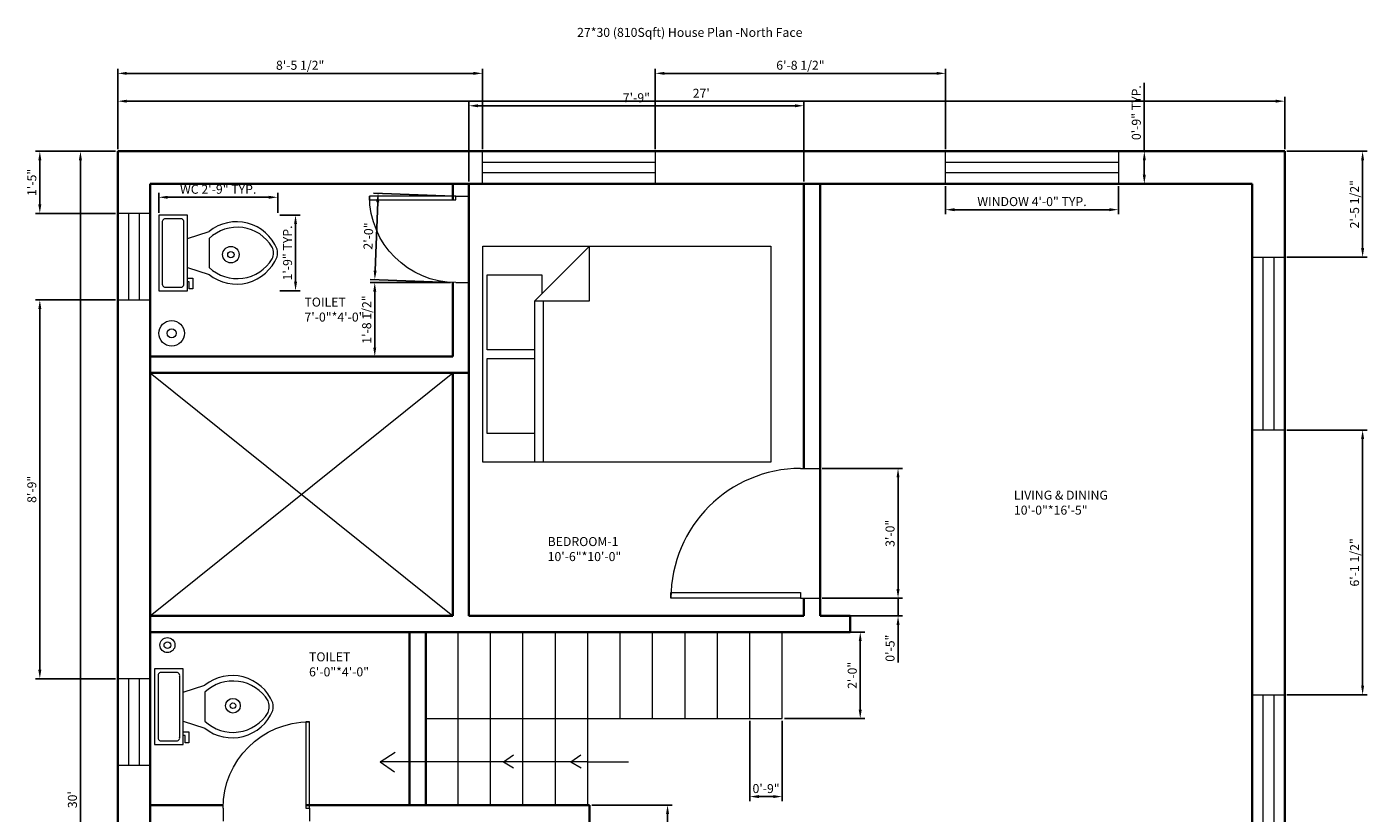
# Model space of a CAD drawing. Units: inches. Extents: x 2721 to 3093, y 1944 to 2371.
# Tile 2 of 2: x 2721 to 3093, y 2152 to 2371. Entities that reach past the tile are written whole.
import ezdxf

# ---------------------------------------------------------------- set-up
doc = ezdxf.new("R2010")
doc.units = ezdxf.units.IN
for name, color, linetype, lineweight in [('A-ANNO-DIMS', 2, 'Continuous', 18), ('A-ANNO-SYMB', 7, 'Continuous', 13), ('A-ANNO-TEXT', 7, 'Continuous', 18), ('A-AREA-IDEN', 7, 'Continuous', 18), ('A-DOOR', 3, 'Continuous', 18), ('A-FLOR-FIXT', 8, 'Continuous', 18), ('A-FLOR-OPEN', 8, 'Continuous', 13), ('A-FLOR-STRS', 7, 'Continuous', 20), ('A-FURN', 9, 'Continuous', 18), ('A-GLAZ', 4, 'Continuous', 18), ('A-WALL', 7, 'Continuous', 35)]:
    doc.layers.add(name, color=color, linetype=linetype, lineweight=lineweight)
doc.styles.get("Standard").update_dxf_attribs({"font": 'arial.ttf'})
doc.dimstyles.new('ISO-25', dxfattribs={"dimtxt": 2.5, "dimasz": 2.5, "dimexe": 1.25, "dimexo": 0.625, "dimtad": 1, "dimdec": 1, "dimlunit": 3, "dimtxsty": 'Standard', "dimcen": 2.5, "dimadec": 0, "dimazin": 0, "dimtfac": 1, "dimtdec": 1, "dimtmove": 0, "dimatfit": 3, "dimfxl": 1, "dimarcsym": 0})

# ---------------------------------------------------------------- blocks, each defined once
blk = doc.blocks.new('*U2')
for p, q in [((0, 0), (0, -6)), ((40, 0), (40, -6))]:
    blk.add_line(p, q)
blk.add_lwpolyline([(0, 0), (0, 40), (1.75, 40), (1.75, 0)], close=True)
blk.add_arc((0, 0), 40, 0, 90)
blk = doc.blocks.new('Bed - Queen')
for p, q in [((0, -80.00003), (0, 0)), ((0, 0), (59.99999, 0)), ((59.99999, 0), (59.99999, -80.00003)), ((7.99999, -1.2), (28.79998, -1.2)), ((7.99999, -14.4), (7.99999, -1.2)), ((28.79998, -1.2), (28.79998, -14.4)), ((31.19999, -1.2), (51.99999, -1.2)), ((31.19999, -14.4), (31.19999, -1.2)), ((51.99999, -1.2), (51.99999, -16.4)), ((0, -14.4), (44.8, -14.4)), ((59.99999, -29.6), (44.8, -14.4)), ((44.8, -14.4), (44.8, -29.6)), ((44.8, -16.8), (0, -16.8)), ((51.99999, -16.4), (46.79936, -16.4)), ((44.8, -29.6), (59.99999, -29.6)), ((59.99999, -80.00003), (0, -80.00003))]:
    blk.add_line(p, q)
blk = doc.blocks.new('Toilet - top')
for p, q in [((9.5, -6), (9.5, -2)), ((-10, -8.5), (-8, -8.5)), ((-10, -9.5), (-10, -8.5)), ((-7, -9.5), (-10, -9.5)), ((-8, -8.5), (-8, -8)), ((-7, -8), (-7, -9.5)), ((-4, -8), (-6, -14)), ((4, -8), (6, -14)), ((4, -14), (-4, -14))]:
    blk.add_line(p, q)
blk.add_lwpolyline([(10.5, -8), (10.5, 0), (-10.5, 0), (-10.5, -8)], close=True)
for points in [[(-9.5, -2), (-9.5, -6)], [(8.5, -1), (-8.5, -1)], [(-8.5, -7), (8.5, -7)]]:
    blk.add_lwpolyline(points)
for centre, radius, start, end in [((-8.62, -1.88), 0.884, 81.8699, 188.1301), ((8.62, -1.88), 0.884, 351.8699, 98.1301), ((-8.62, -6.12), 0.884, 171.8699, 278.1301), ((8.62, -6.12), 0.884, 261.8699, 8.1301), ((3.52, -21.58), 12.17, 141.4691, 247.9714), ((4.2, -21.82), 11.33, 136.3677, 238.9468), ((-3.52, -21.58), 12.17, 292.0284, 38.5307), ((-4.2, -21.82), 11.33, 301.053, 43.6321), ((0, -27.88), 4, 245.7318, 294.2682), ((0, -29), 4, 254.8605, 285.1395)]:
    blk.add_arc(centre, radius, start, end)
blk = doc.blocks.new('*D6')
at = {"layer": 'A-ANNO-DIMS', "color": 0, "lineweight": -2, "transparency": 16777216}
for p, q in [((2745.8, 2336.8), (2745.8, 2351.35)), ((2748.3, 2350.1), (3067.3, 2350.1)), ((3069.8, 2336.8), (3069.8, 2351.35))]:
    blk.add_line(p, q, dxfattribs=at)
at = {"layer": 'A-ANNO-DIMS', "color": 0, "transparency": 16777216}
for points in [[(2748.3, 2350.52), (2748.3, 2349.69), (2745.8, 2350.1)], [(3067.3, 2350.52), (3067.3, 2349.69), (3069.8, 2350.1)]]:
    blk.add_solid(points, dxfattribs=at)
at = {"layer": 'Defpoints', "color": 0, "transparency": 16777216}
for p in [(3069.8, 2350.1), (2745.8, 2336.18), (3069.8, 2336.18)]:
    blk.add_point(p, dxfattribs=at)
at = {"layer": 'A-ANNO-DIMS', "color": 0, "transparency": 16777216, "insert": (2907.8, 2351.98), "char_height": 2.5, "attachment_point": 5}
blk.add_mtext("27'", dxfattribs=at)
blk = doc.blocks.new('*D7')
at = {"layer": 'A-ANNO-DIMS', "color": 0, "lineweight": -2, "transparency": 16777216}
for p, q in [((2745.17, 2336.18), (2734.17, 2336.18)), ((2735.42, 2333.68), (2735.42, 1978.68)), ((2745.17, 1976.18), (2734.17, 1976.18))]:
    blk.add_line(p, q, dxfattribs=at)
at = {"layer": 'A-ANNO-DIMS', "color": 0, "transparency": 16777216}
for points in [[(2735, 2333.68), (2735.84, 2333.68), (2735.42, 2336.18)], [(2735, 1978.68), (2735.84, 1978.68), (2735.42, 1976.18)]]:
    blk.add_solid(points, dxfattribs=at)
at = {"layer": 'Defpoints', "color": 0, "transparency": 16777216}
for p in [(2745.8, 2336.18), (2735.42, 1976.18), (2745.8, 1976.18)]:
    blk.add_point(p, dxfattribs=at)
at = {"layer": 'A-ANNO-DIMS', "color": 0, "transparency": 16777216, "insert": (2733.52, 2156.18), "char_height": 2.5, "attachment_point": 5, "rotation": 90}
blk.add_mtext("30'", dxfattribs=at)
blk = doc.blocks.new('WIN-48IN')
for p, q in [((0, 9), (48, 9)), ((0, 0), (0, 9)), ((48, 9), (48, 0)), ((0, 6), (48, 6)), ((48, 3), (0, 3)), ((48, 0), (0, 0))]:
    blk.add_line(p, q)
blk = doc.blocks.new('WIN-24IN')
for p, q in [((9, 24), (0, 24)), ((0, 24), (0, 0)), ((3, 24), (3, 0)), ((6, 0), (6, 24)), ((9, 0), (9, 24)), ((0, 0), (9, 0))]:
    blk.add_line(p, q)
blk = doc.blocks.new('*D11')
at = {"layer": 'A-ANNO-DIMS', "color": 0, "lineweight": -2, "transparency": 16777216}
for p, q in [((2975.63, 2326.55), (2975.63, 2318.73)), ((3023.63, 2326.55), (3023.63, 2318.73)), ((2978.13, 2319.98), (3021.13, 2319.98))]:
    blk.add_line(p, q, dxfattribs=at)
at = {"layer": 'A-ANNO-DIMS', "color": 0, "transparency": 16777216}
for points in [[(2978.13, 2320.39), (2978.13, 2319.56), (2975.63, 2319.98)], [(3021.13, 2320.39), (3021.13, 2319.56), (3023.63, 2319.98)]]:
    blk.add_solid(points, dxfattribs=at)
at = {"layer": 'Defpoints', "color": 0, "transparency": 16777216}
for p in [(2975.63, 2327.18), (3023.63, 2327.18), (3023.63, 2319.98)]:
    blk.add_point(p, dxfattribs=at)
at = {"layer": 'A-ANNO-DIMS', "color": 0, "transparency": 16777216, "insert": (2999.63, 2321.9), "char_height": 2.5, "attachment_point": 5}
blk.add_mtext('WINDOW 4\'-0" TYP.', dxfattribs=at)
blk = doc.blocks.new('*D12')
at = {"layer": 'A-ANNO-DIMS', "color": 0, "lineweight": -2, "transparency": 16777216}
for p, q in [((3030.83, 2336.18), (3030.83, 2355.17)), ((3024.26, 2336.18), (3032.08, 2336.18)), ((3030.83, 2329.68), (3030.83, 2333.68)), ((3024.26, 2327.18), (3032.08, 2327.18))]:
    blk.add_line(p, q, dxfattribs=at)
at = {"layer": 'A-ANNO-DIMS', "color": 0, "transparency": 16777216}
for points in [[(3030.41, 2333.68), (3031.25, 2333.68), (3030.83, 2336.18)], [(3030.41, 2329.68), (3031.25, 2329.68), (3030.83, 2327.18)]]:
    blk.add_solid(points, dxfattribs=at)
at = {"layer": 'Defpoints', "color": 0, "transparency": 16777216}
for p in [(3023.63, 2336.18), (3030.83, 2336.18), (3023.63, 2327.18)]:
    blk.add_point(p, dxfattribs=at)
at = {"layer": 'A-ANNO-DIMS', "color": 0, "transparency": 16777216, "insert": (3028.93, 2346.92), "char_height": 2.5, "attachment_point": 5, "rotation": 90}
blk.add_mtext('0\'-9" TYP.', dxfattribs=at)
blk = doc.blocks.new('*D17')
at = {"layer": 'A-ANNO-DIMS', "color": 0, "lineweight": -2, "transparency": 16777216}
for p, q in [((2757.15, 2319.09), (2757.15, 2324.67)), ((2787.69, 2323.42), (2759.65, 2323.42)), ((2790.19, 2319.09), (2790.19, 2324.67))]:
    blk.add_line(p, q, dxfattribs=at)
at = {"layer": 'A-ANNO-DIMS', "color": 0, "transparency": 16777216}
for points in [[(2759.65, 2323.83), (2759.65, 2323), (2757.15, 2323.42)], [(2787.69, 2323.83), (2787.69, 2323), (2790.19, 2323.42)]]:
    blk.add_solid(points, dxfattribs=at)
at = {"layer": 'Defpoints', "color": 0, "transparency": 16777216}
for p in [(2757.15, 2323.42), (2757.15, 2318.46), (2790.19, 2318.46)]:
    blk.add_point(p, dxfattribs=at)
at = {"layer": 'A-ANNO-DIMS', "color": 0, "transparency": 16777216, "insert": (2773.67, 2325.33), "char_height": 2.5, "attachment_point": 5}
blk.add_mtext('WC 2\'-9" TYP.', dxfattribs=at)
blk = doc.blocks.new('*D18')
at = {"layer": 'A-ANNO-DIMS', "color": 0, "lineweight": -2, "transparency": 16777216}
for p, q in [((2790.82, 2318.46), (2796.4, 2318.46)), ((2795.15, 2299.96), (2795.15, 2315.96)), ((2790.82, 2297.46), (2796.4, 2297.46))]:
    blk.add_line(p, q, dxfattribs=at)
at = {"layer": 'A-ANNO-DIMS', "color": 0, "transparency": 16777216}
for points in [[(2794.74, 2315.96), (2795.57, 2315.96), (2795.15, 2318.46)], [(2794.74, 2299.96), (2795.57, 2299.96), (2795.15, 2297.46)]]:
    blk.add_solid(points, dxfattribs=at)
at = {"layer": 'Defpoints', "color": 0, "transparency": 16777216}
for p in [(2790.19, 2318.46), (2795.15, 2318.46), (2790.19, 2297.46)]:
    blk.add_point(p, dxfattribs=at)
at = {"layer": 'A-ANNO-DIMS', "color": 0, "transparency": 16777216, "insert": (2793.25, 2307.96), "char_height": 2.5, "attachment_point": 5, "rotation": 90}
blk.add_mtext('1\'-9" TYP.', dxfattribs=at)
blk = doc.blocks.new('*D23')
at = {"layer": 'A-ANNO-DIMS', "color": 0, "lineweight": -2, "transparency": 16777216}
for p, q in [((2745.8, 2336.8), (2745.8, 2359.08)), ((2748.3, 2357.83), (2844.55, 2357.83)), ((2847.05, 2336.8), (2847.05, 2359.08))]:
    blk.add_line(p, q, dxfattribs=at)
at = {"layer": 'A-ANNO-DIMS', "color": 0, "transparency": 16777216}
for points in [[(2748.3, 2358.24), (2748.3, 2357.41), (2745.8, 2357.83)], [(2844.55, 2358.24), (2844.55, 2357.41), (2847.05, 2357.83)]]:
    blk.add_solid(points, dxfattribs=at)
at = {"layer": 'Defpoints', "color": 0, "transparency": 16777216}
for p in [(2847.05, 2357.83), (2745.8, 2336.18), (2847.05, 2336.18)]:
    blk.add_point(p, dxfattribs=at)
at = {"layer": 'A-ANNO-DIMS', "color": 0, "transparency": 16777216, "insert": (2796.43, 2359.75), "char_height": 2.5, "attachment_point": 5}
blk.add_mtext('8\'-5 1/2"', dxfattribs=at)
blk = doc.blocks.new('*D24')
at = {"layer": 'A-ANNO-DIMS', "color": 0, "lineweight": -2, "transparency": 16777216}
for p, q in [((2895.05, 2336.8), (2895.05, 2359.08)), ((2897.55, 2357.83), (2973.13, 2357.83)), ((2975.63, 2336.8), (2975.63, 2359.08))]:
    blk.add_line(p, q, dxfattribs=at)
at = {"layer": 'A-ANNO-DIMS', "color": 0, "transparency": 16777216}
for points in [[(2897.55, 2358.24), (2897.55, 2357.41), (2895.05, 2357.83)], [(2973.13, 2358.24), (2973.13, 2357.41), (2975.63, 2357.83)]]:
    blk.add_solid(points, dxfattribs=at)
at = {"layer": 'Defpoints', "color": 0, "transparency": 16777216}
for p in [(2975.63, 2357.83), (2895.05, 2336.18), (2975.63, 2336.18)]:
    blk.add_point(p, dxfattribs=at)
at = {"layer": 'A-ANNO-DIMS', "color": 0, "transparency": 16777216, "insert": (2935.34, 2359.75), "char_height": 2.5, "attachment_point": 5}
blk.add_mtext('6\'-8 1/2"', dxfattribs=at)
blk = doc.blocks.new('*D28')
at = {"layer": 'A-ANNO-DIMS', "color": 0, "lineweight": -2, "transparency": 16777216}
for p, q in [((2745.17, 2336.18), (2722.9, 2336.18)), ((2724.15, 2321.43), (2724.15, 2333.68)), ((2745.17, 2318.93), (2722.9, 2318.93))]:
    blk.add_line(p, q, dxfattribs=at)
at = {"layer": 'A-ANNO-DIMS', "color": 0, "transparency": 16777216}
for points in [[(2723.73, 2333.68), (2724.56, 2333.68), (2724.15, 2336.18)], [(2723.73, 2321.43), (2724.56, 2321.43), (2724.15, 2318.93)]]:
    blk.add_solid(points, dxfattribs=at)
at = {"layer": 'Defpoints', "color": 0, "transparency": 16777216}
for p in [(2724.15, 2336.18), (2745.8, 2336.18), (2745.8, 2318.93)]:
    blk.add_point(p, dxfattribs=at)
at = {"layer": 'A-ANNO-DIMS', "color": 0, "transparency": 16777216, "insert": (2722.25, 2327.56), "char_height": 2.5, "attachment_point": 5, "rotation": 90}
blk.add_mtext('1\'-5"', dxfattribs=at)
blk = doc.blocks.new('*D29')
at = {"layer": 'A-ANNO-DIMS', "color": 0, "lineweight": -2, "transparency": 16777216}
for p, q in [((2745.17, 2294.93), (2722.9, 2294.93)), ((2724.15, 2192.23), (2724.15, 2292.43)), ((2745.17, 2189.73), (2722.9, 2189.73))]:
    blk.add_line(p, q, dxfattribs=at)
at = {"layer": 'A-ANNO-DIMS', "color": 0, "transparency": 16777216}
for points in [[(2723.73, 2292.43), (2724.56, 2292.43), (2724.15, 2294.93)], [(2723.73, 2192.23), (2724.56, 2192.23), (2724.15, 2189.73)]]:
    blk.add_solid(points, dxfattribs=at)
at = {"layer": 'Defpoints', "color": 0, "transparency": 16777216}
for p in [(2724.15, 2294.93), (2745.8, 2294.93), (2745.8, 2189.73)]:
    blk.add_point(p, dxfattribs=at)
at = {"layer": 'A-ANNO-DIMS', "color": 0, "transparency": 16777216, "insert": (2722.25, 2242.33), "char_height": 2.5, "attachment_point": 5, "rotation": 90}
blk.add_mtext('8\'-9"', dxfattribs=at)
blk = doc.blocks.new('*D30')
at = {"layer": 'A-ANNO-DIMS', "color": 0, "lineweight": -2, "transparency": 16777216}
for p, q in [((3070.42, 2336.18), (3092.7, 2336.18)), ((3091.45, 2333.68), (3091.45, 2309.3)), ((3070.42, 2306.8), (3092.7, 2306.8))]:
    blk.add_line(p, q, dxfattribs=at)
at = {"layer": 'A-ANNO-DIMS', "color": 0, "transparency": 16777216}
for points in [[(3091.03, 2333.68), (3091.86, 2333.68), (3091.45, 2336.18)], [(3091.03, 2309.3), (3091.86, 2309.3), (3091.45, 2306.8)]]:
    blk.add_solid(points, dxfattribs=at)
at = {"layer": 'Defpoints', "color": 0, "transparency": 16777216}
for p in [(3069.8, 2336.18), (3069.8, 2306.8), (3091.45, 2306.8)]:
    blk.add_point(p, dxfattribs=at)
at = {"layer": 'A-ANNO-DIMS', "color": 0, "transparency": 16777216, "insert": (3089.53, 2321.49), "char_height": 2.5, "attachment_point": 5, "rotation": 90}
blk.add_mtext('2\'-5 1/2"', dxfattribs=at)
blk = doc.blocks.new('*D31')
at = {"layer": 'A-ANNO-DIMS', "color": 0, "lineweight": -2, "transparency": 16777216}
for p, q in [((3070.42, 2258.8), (3092.7, 2258.8)), ((3091.45, 2256.3), (3091.45, 2187.81)), ((3070.42, 2185.31), (3092.7, 2185.31))]:
    blk.add_line(p, q, dxfattribs=at)
at = {"layer": 'A-ANNO-DIMS', "color": 0, "transparency": 16777216}
for points in [[(3091.03, 2256.3), (3091.86, 2256.3), (3091.45, 2258.8)], [(3091.03, 2187.81), (3091.86, 2187.81), (3091.45, 2185.31)]]:
    blk.add_solid(points, dxfattribs=at)
at = {"layer": 'Defpoints', "color": 0, "transparency": 16777216}
for p in [(3069.8, 2258.8), (3069.8, 2185.31), (3091.45, 2185.31)]:
    blk.add_point(p, dxfattribs=at)
at = {"layer": 'A-ANNO-DIMS', "color": 0, "transparency": 16777216, "insert": (3089.53, 2222.05), "char_height": 2.5, "attachment_point": 5, "rotation": 90}
blk.add_mtext('6\'-1 1/2"', dxfattribs=at)
blk = doc.blocks.new('*D34')
at = {"layer": 'A-ANNO-DIMS', "color": 0, "lineweight": -2, "transparency": 16777216}
for p, q in [((2930.92, 2202.68), (2953.2, 2202.68)), ((2951.95, 2200.18), (2951.95, 2181.18)), ((2930.92, 2178.68), (2953.2, 2178.68))]:
    blk.add_line(p, q, dxfattribs=at)
at = {"layer": 'A-ANNO-DIMS', "color": 0, "transparency": 16777216}
for points in [[(2951.53, 2200.18), (2952.36, 2200.18), (2951.95, 2202.68)], [(2951.53, 2181.18), (2952.36, 2181.18), (2951.95, 2178.68)]]:
    blk.add_solid(points, dxfattribs=at)
at = {"layer": 'Defpoints', "color": 0, "transparency": 16777216}
for p in [(2930.3, 2202.68), (2930.3, 2178.68), (2951.95, 2178.68)]:
    blk.add_point(p, dxfattribs=at)
at = {"layer": 'A-ANNO-DIMS', "color": 0, "transparency": 16777216, "insert": (2950.05, 2190.68), "char_height": 2.5, "attachment_point": 5, "rotation": 90}
blk.add_mtext('2\'-0"', dxfattribs=at)
blk = doc.blocks.new('*D35')
at = {"layer": 'A-ANNO-DIMS', "color": 0, "lineweight": -2, "transparency": 16777216}
for p, q in [((2921.3, 2178.05), (2921.3, 2155.78)), ((2930.3, 2178.05), (2930.3, 2155.78)), ((2927.8, 2157.03), (2923.8, 2157.03))]:
    blk.add_line(p, q, dxfattribs=at)
at = {"layer": 'A-ANNO-DIMS', "color": 0, "transparency": 16777216}
for points in [[(2923.8, 2157.44), (2923.8, 2156.61), (2921.3, 2157.03)], [(2927.8, 2157.44), (2927.8, 2156.61), (2930.3, 2157.03)]]:
    blk.add_solid(points, dxfattribs=at)
at = {"layer": 'Defpoints', "color": 0, "transparency": 16777216}
for p in [(2921.3, 2178.68), (2930.3, 2178.68), (2921.3, 2157.03)]:
    blk.add_point(p, dxfattribs=at)
at = {"layer": 'A-ANNO-DIMS', "color": 0, "transparency": 16777216, "insert": (2925.8, 2158.93), "char_height": 2.5, "attachment_point": 5}
blk.add_mtext('0\'-9"', dxfattribs=at)
blk = doc.blocks.new('*D36')
at = {"layer": 'A-ANNO-DIMS', "color": 0, "lineweight": -2, "transparency": 16777216}
for p, q in [((2941.42, 2248.12), (2963.7, 2248.12)), ((2962.45, 2245.62), (2962.45, 2214.62)), ((2941.42, 2212.12), (2963.7, 2212.12))]:
    blk.add_line(p, q, dxfattribs=at)
at = {"layer": 'A-ANNO-DIMS', "color": 0, "transparency": 16777216}
for points in [[(2962.03, 2245.62), (2962.86, 2245.62), (2962.45, 2248.12)], [(2962.03, 2214.62), (2962.86, 2214.62), (2962.45, 2212.12)]]:
    blk.add_solid(points, dxfattribs=at)
at = {"layer": 'Defpoints', "color": 0, "transparency": 16777216}
for p in [(2940.8, 2248.12), (2940.8, 2212.12), (2962.45, 2212.12)]:
    blk.add_point(p, dxfattribs=at)
at = {"layer": 'A-ANNO-DIMS', "color": 0, "transparency": 16777216, "insert": (2960.55, 2230.12), "char_height": 2.5, "attachment_point": 5, "rotation": 90}
blk.add_mtext('3\'-0"', dxfattribs=at)
blk = doc.blocks.new('*D43')
at = {"layer": 'A-ANNO-DIMS', "color": 0, "lineweight": -2, "transparency": 16777216}
for p, q in [((2839.07, 2323.76), (2816.81, 2324.6)), ((2817.26, 2303.06), (2817.97, 2322.05)), ((2838.17, 2299.78), (2815.91, 2300.61))]:
    blk.add_line(p, q, dxfattribs=at)
at = {"layer": 'A-ANNO-DIMS', "color": 0, "transparency": 16777216}
for points in [[(2817.55, 2322.07), (2818.39, 2322.04), (2818.06, 2324.55)], [(2816.84, 2303.08), (2817.67, 2303.05), (2817.16, 2300.57)]]:
    blk.add_solid(points, dxfattribs=at)
at = {"layer": 'Defpoints', "color": 0, "transparency": 16777216}
for p in [(2818.06, 2324.55), (2839.7, 2323.74), (2838.8, 2299.75)]:
    blk.add_point(p, dxfattribs=at)
at = {"layer": 'A-ANNO-DIMS', "color": 0, "transparency": 16777216, "insert": (2815.71, 2312.63), "char_height": 2.5, "attachment_point": 5, "rotation": 87.8509}
blk.add_mtext('2\'-0"', dxfattribs=at)
blk = doc.blocks.new('*D44')
at = {"layer": 'A-ANNO-DIMS', "color": 0, "lineweight": -2, "transparency": 16777216}
for p, q in [((2838.17, 2299.75), (2815.9, 2299.75)), ((2817.15, 2281.68), (2817.15, 2297.25)), ((2838.17, 2279.18), (2815.9, 2279.18))]:
    blk.add_line(p, q, dxfattribs=at)
at = {"layer": 'A-ANNO-DIMS', "color": 0, "transparency": 16777216}
for points in [[(2816.73, 2297.25), (2817.56, 2297.25), (2817.15, 2299.75)], [(2816.73, 2281.68), (2817.56, 2281.68), (2817.15, 2279.18)]]:
    blk.add_solid(points, dxfattribs=at)
at = {"layer": 'Defpoints', "color": 0, "transparency": 16777216}
for p in [(2817.15, 2299.75), (2838.8, 2299.75), (2838.8, 2279.18)]:
    blk.add_point(p, dxfattribs=at)
at = {"layer": 'A-ANNO-DIMS', "color": 0, "transparency": 16777216, "insert": (2815.23, 2289.47), "char_height": 2.5, "attachment_point": 5, "rotation": 90}
blk.add_mtext('1\'-8 1/2"', dxfattribs=at)
blk = doc.blocks.new('*D45')
at = {"layer": 'A-ANNO-DIMS', "color": 0, "lineweight": -2, "transparency": 16777216}
for p, q in [((2962.45, 2214.62), (2962.45, 2217.12)), ((2941.42, 2212.12), (2963.7, 2212.12)), ((2962.45, 2212.12), (2962.45, 2207.18)), ((2941.42, 2207.18), (2963.7, 2207.18)), ((2962.45, 2204.68), (2962.45, 2194.28))]:
    blk.add_line(p, q, dxfattribs=at)
at = {"layer": 'A-ANNO-DIMS', "color": 0, "transparency": 16777216}
for points in [[(2962.03, 2214.62), (2962.86, 2214.62), (2962.45, 2212.12)], [(2962.03, 2204.68), (2962.86, 2204.68), (2962.45, 2207.18)]]:
    blk.add_solid(points, dxfattribs=at)
at = {"layer": 'Defpoints', "color": 0, "transparency": 16777216}
for p in [(2940.8, 2212.12), (2940.8, 2207.18), (2962.45, 2207.18)]:
    blk.add_point(p, dxfattribs=at)
at = {"layer": 'A-ANNO-DIMS', "color": 0, "transparency": 16777216, "insert": (2960.55, 2198.23), "char_height": 2.5, "attachment_point": 5, "rotation": 90}
blk.add_mtext('0\'-5"', dxfattribs=at)
blk = doc.blocks.new('*D46')
at = {"layer": 'A-ANNO-DIMS', "color": 0, "lineweight": -2, "transparency": 16777216}
for p, q in [((2877.42, 2154.68), (2899.7, 2154.68)), ((2898.45, 2152.18), (2898.45, 2147.68)), ((2877.42, 2145.18), (2899.7, 2145.18)), ((2898.45, 2145.18), (2898.45, 2128.96))]:
    blk.add_line(p, q, dxfattribs=at)
at = {"layer": 'A-ANNO-DIMS', "color": 0, "transparency": 16777216}
for points in [[(2898.03, 2152.18), (2898.86, 2152.18), (2898.45, 2154.68)], [(2898.03, 2147.68), (2898.86, 2147.68), (2898.45, 2145.18)]]:
    blk.add_solid(points, dxfattribs=at)
at = {"layer": 'Defpoints', "color": 0, "transparency": 16777216}
for p in [(2876.8, 2154.68), (2876.8, 2145.18), (2898.45, 2145.18)]:
    blk.add_point(p, dxfattribs=at)
at = {"layer": 'A-ANNO-DIMS', "color": 0, "transparency": 16777216, "insert": (2896.53, 2135.82), "char_height": 2.5, "attachment_point": 5, "rotation": 90}
blk.add_mtext('0\'-9 1/2"', dxfattribs=at)
blk = doc.blocks.new('*D49')
at = {"layer": 'A-ANNO-DIMS', "color": 0, "lineweight": -2, "transparency": 16777216}
for p, q in [((2843.3, 2327.8), (2843.3, 2350.08)), ((2845.8, 2348.83), (2933.8, 2348.83)), ((2936.3, 2327.8), (2936.3, 2350.08))]:
    blk.add_line(p, q, dxfattribs=at)
at = {"layer": 'A-ANNO-DIMS', "color": 0, "transparency": 16777216}
for points in [[(2845.8, 2349.24), (2845.8, 2348.41), (2843.3, 2348.83)], [(2933.8, 2349.24), (2933.8, 2348.41), (2936.3, 2348.83)]]:
    blk.add_solid(points, dxfattribs=at)
at = {"layer": 'Defpoints', "color": 0, "transparency": 16777216}
for p in [(2936.3, 2348.83), (2843.3, 2327.18), (2936.3, 2327.18)]:
    blk.add_point(p, dxfattribs=at)
at = {"layer": 'A-ANNO-DIMS', "color": 0, "transparency": 16777216, "insert": (2889.8, 2350.73), "char_height": 2.5, "attachment_point": 5}
blk.add_mtext('7\'-9"', dxfattribs=at)

msp = doc.modelspace()

# ---------------------------------------------------------------- linework, layer by layer
at = {"layer": 'A-ANNO-SYMB'}
for p, q in [((2818.66, 2166.68), (2822.83, 2169.35)), ((2876.3, 2166.68), (2818.66, 2166.68)), ((2818.66, 2166.68), (2822.63, 2163.9)), ((2852.92, 2166.68), (2855.68, 2168.64)), ((2852.92, 2166.68), (2855.68, 2165.04)), ((2871.59, 2166.68), (2874.34, 2168.59)), ((2871.59, 2166.68), (2874.47, 2165.02)), ((2876.3, 2166.68), (2887.63, 2166.68))]:
    msp.add_line(p, q, dxfattribs=at)
at = {"layer": 'A-FLOR-FIXT'}
for centre, radius in [((2777.2, 2307.5), 2.29), ((2777.2, 2307.5), 0.886), ((2760.74, 2285.65), 3.55), ((2760.74, 2285.65), 1.28), ((2759.57, 2199.09), 2.09), ((2759.57, 2199.09), 0.925), ((2777.78, 2182.26), 2.04), ((2777.78, 2182.26), 0.773)]:
    msp.add_circle(centre, radius, dxfattribs=at)
at = {"layer": 'A-FLOR-OPEN'}
for p, q in [((2754.8, 2274.68), (2838.8, 2207.18)), ((2754.8, 2207.18), (2838.8, 2274.68))]:
    msp.add_line(p, q, dxfattribs=at)
at = {"layer": 'A-FLOR-STRS'}
for p, q in [((2840.3, 2154.68), (2840.3, 2202.68)), ((2849.3, 2154.68), (2849.3, 2202.68)), ((2858.3, 2154.68), (2858.3, 2202.68)), ((2867.3, 2154.68), (2867.3, 2202.68)), ((2876.3, 2154.68), (2876.3, 2202.68)), ((2885.3, 2178.68), (2885.3, 2202.68)), ((2894.3, 2178.68), (2894.3, 2202.68)), ((2903.3, 2178.68), (2903.3, 2202.68)), ((2912.3, 2178.68), (2912.3, 2202.68)), ((2921.3, 2178.68), (2921.3, 2202.68)), ((2930.3, 2178.68), (2930.3, 2202.68)), ((2831.3, 2178.68), (2930.3, 2178.68))]:
    msp.add_line(p, q, dxfattribs=at)
at = {"layer": 'A-WALL'}
for p, q in [((2745.8, 2336.18), (3069.8, 2336.18)), ((2745.8, 1976.18), (2745.8, 2336.18)), ((3069.8, 2336.18), (3069.8, 1976.18)), ((2754.8, 2327.18), (3060.8, 2327.18)), ((2754.8, 1985.18), (2754.8, 2327.18)), ((2838.8, 2322.69), (2838.8, 2327.18)), ((2843.3, 2207.18), (2843.3, 2327.18)), ((2936.3, 2327.18), (2936.3, 2248.12)), ((2940.8, 2327.18), (2940.8, 2207.18)), ((3060.8, 2327.18), (3060.8, 2130.18)), ((2838.8, 2279.18), (2838.8, 2299.75)), ((2754.8, 2279.18), (2838.8, 2279.18)), ((2754.8, 2274.68), (2843.3, 2274.68)), ((2838.8, 2207.18), (2838.8, 2274.68)), ((2936.3, 2212.12), (2936.3, 2207.18)), ((2754.8, 2207.18), (2838.8, 2207.18)), ((2843.3, 2207.18), (2936.3, 2207.18)), ((2940.8, 2207.18), (2949.18, 2207.18)), ((2949.18, 2202.68), (2949.18, 2207.18)), ((2754.8, 2202.68), (2940.8, 2202.68)), ((2826.8, 2154.68), (2826.8, 2202.68)), ((2831.3, 2154.68), (2831.3, 2202.68)), ((2940.8, 2202.68), (2949.18, 2202.68)), ((2754.8, 2154.68), (2775.04, 2154.68)), ((2797.98, 2154.68), (2876.8, 2154.68)), ((2876.8, 2154.68), (2876.8, 1985.18))]:
    msp.add_line(p, q, dxfattribs=at)

# ---------------------------------------------------------------- block references
at = {"layer": 'A-DOOR'}
for p, xscale, yscale, zscale, rotation in [((2839.7, 2323.74), -0.6, 0.6, 0.6, 90), ((2935.4, 2212.12), 0.9, 0.9, 0.9, 90.00000000000003)]:
    msp.add_blockref('*U2', p, dxfattribs=dict(at, xscale=xscale, yscale=yscale, zscale=zscale, rotation=rotation))
at = {"layer": 'A-DOOR', "xscale": -0.6, "yscale": 0.6, "zscale": 0.6}
msp.add_blockref('*U2', (2799.03, 2153.78), dxfattribs=at)
at = {"layer": 'A-FLOR-FIXT', "rotation": 90}
for p in [(2757.15, 2307.96), (2755.98, 2181.99)]:
    msp.add_blockref('Toilet - top', p, dxfattribs=at)
at = {"layer": 'A-FURN', "rotation": 90}
msp.add_blockref('Bed - Queen', (2847.15, 2249.87), dxfattribs=at)
at = {"layer": 'A-GLAZ'}
for name, p in [('WIN-48IN', (2847.05, 2327.18)), ('WIN-48IN', (2975.63, 2327.18)), ('WIN-24IN', (2745.8, 2294.93)), ('WIN-24IN', (2745.8, 2165.73))]:
    msp.add_blockref(name, p, dxfattribs=at)
for p, rotation in [((3069.8, 2258.8), 90.00000000000317), ((3069.8, 2137.31), 90.00000000000276)]:
    msp.add_blockref('WIN-48IN', p, dxfattribs=dict(at, rotation=rotation))

# ---------------------------------------------------------------- texts
at = {"layer": 'A-ANNO-TEXT', "insert": (2873.33, 2370.45), "char_height": 2.5, "attachment_point": 1}
msp.add_mtext_dynamic_manual_height_columns('27*30 (810Sqft) House Plan -North Face', width=309.6567, gutter_width=12.5, heights=[0], dxfattribs=at)
at = {"layer": 'A-AREA-IDEN', "char_height": 2.5, "attachment_point": 1}
for s, width, insert in [('TOILET\\P7\'-0"*4\'-0"', 45.6593, (2797.63, 2295.57)), ('LIVING & DINING\\P10\'-0"*16\'-5"', 53.9387, (2994.62, 2241.97)), ('BEDROOM-1\\P10\'-6"*10\'-0"', 36.6403, (2865.15, 2229.08)), ('TOILET\\P6\'-0"*4\'-0"', 29.6279, (2798.9, 2197.07))]:
    msp.add_mtext_dynamic_manual_height_columns(s, width=width, gutter_width=12.5, heights=[0], dxfattribs=dict(at, insert=insert))

# ---------------------------------------------------------------- dimensions: what is measured, and where the dimension line sits
at = {"layer": 'A-ANNO-DIMS'}
for base, p1, p2, angle, override, picture, middle in [((2847.054, 2357.8275), (2745.7983, 2336.1775), (2847.054, 2336.1775), 0, {"dimdec": 1, "dimlfac": 1, "dimrnd": 0, "dimzin": 1, "dimdsep": 46, "dimlunit": 4, "dimfrac": 2}, '*D23', (2796.4262, 2359.7451)), ((2724.1483, 2336.1775), (2745.7983, 2318.9347), (2745.7983, 2336.1775), 90, {"dimdec": 1, "dimlfac": 1, "dimrnd": 0, "dimzin": 1, "dimdsep": 46, "dimlunit": 4, "dimfrac": 2}, '*D28', (2722.2469, 2327.5561)), ((2735.42, 1976.18), (2745.8, 2336.18), (2745.8, 1976.18), 90, {"dimclrd": 0, "dimclre": 0, "dimclrt": 0}, '*D7', (2733.52, 2156.18)), ((3091.45, 2306.8), (3069.8, 2336.18), (3069.8, 2306.8), 270, {"dimdec": 1, "dimlfac": 1, "dimrnd": 0, "dimzin": 1, "dimdsep": 46, "dimlunit": 4, "dimfrac": 2}, '*D30', (3089.53, 2321.49)), ((2818.06, 2324.55), (2838.8, 2299.75), (2839.7, 2323.74), 87.8509, {"dimdec": 1, "dimlfac": 1, "dimrnd": 0, "dimzin": 1, "dimdsep": 46, "dimlunit": 4, "dimfrac": 2}, '*D43', (2815.71, 2312.63)), ((2817.15, 2299.75), (2838.8, 2279.18), (2838.8, 2299.75), 90, {"dimdec": 1, "dimlfac": 1, "dimrnd": 0, "dimzin": 1, "dimdsep": 46, "dimlunit": 4, "dimfrac": 2}, '*D44', (2815.23, 2289.47)), ((2724.15, 2294.93), (2745.8, 2189.73), (2745.8, 2294.93), 90, {"dimdec": 1, "dimlfac": 1, "dimrnd": 0, "dimzin": 1, "dimdsep": 46, "dimlunit": 4, "dimfrac": 2}, '*D29', (2722.25, 2242.33)), ((3091.45, 2185.31), (3069.8, 2258.8), (3069.8, 2185.31), 270, {"dimdec": 1, "dimlfac": 1, "dimrnd": 0, "dimzin": 1, "dimdsep": 46, "dimlunit": 4, "dimfrac": 2}, '*D31', (3089.53, 2222.05)), ((2962.45, 2212.12), (2940.8, 2248.12), (2940.8, 2212.12), 270, {"dimdec": 1, "dimlfac": 1, "dimrnd": 0, "dimzin": 1, "dimdsep": 46, "dimlunit": 4, "dimfrac": 2}, '*D36', (2960.55, 2230.12)), ((2962.45, 2207.18), (2940.8, 2212.12), (2940.8, 2207.18), 270, {"dimdec": 1, "dimlfac": 1, "dimrnd": 0, "dimzin": 1, "dimdsep": 46, "dimlunit": 4, "dimfrac": 2}, '*D45', (2960.55, 2198.23)), ((2951.95, 2178.68), (2930.3, 2202.68), (2930.3, 2178.68), 270, {"dimdec": 1, "dimlfac": 1, "dimrnd": 0, "dimzin": 1, "dimdsep": 46, "dimlunit": 4, "dimfrac": 2}, '*D34', (2950.05, 2190.68)), ((2921.3, 2157.03), (2930.3, 2178.68), (2921.3, 2178.68), 180, {"dimdec": 1, "dimlfac": 1, "dimrnd": 0, "dimzin": 1, "dimdsep": 46, "dimlunit": 4, "dimfrac": 2}, '*D35', (2925.8, 2158.93)), ((2898.45, 2145.18), (2876.8, 2154.68), (2876.8, 2145.18), 270, {"dimdec": 1, "dimlfac": 1, "dimrnd": 0, "dimzin": 1, "dimdsep": 46, "dimlunit": 4, "dimfrac": 2}, '*D46', (2896.53, 2135.82))]:
    dim = msp.add_linear_dim(base=base, p1=p1, p2=p2, angle=angle, dimstyle='ISO-25', override=override, dxfattribs=at)
    dim.commit()
    dim.dimension.update_dxf_attribs({"geometry": picture, "text_midpoint": middle})
for base, p1, p2, override, picture, middle in [((2975.63, 2357.83), (2895.05, 2336.18), (2975.63, 2336.18), {"dimdec": 1, "dimlfac": 1, "dimrnd": 0, "dimzin": 1, "dimdsep": 46, "dimlunit": 4, "dimfrac": 2}, '*D24', (2935.34, 2359.75)), ((3069.8, 2350.1), (2745.8, 2336.18), (3069.8, 2336.18), {"dimclrd": 0, "dimclre": 0, "dimclrt": 0}, '*D6', (2907.8, 2351.98)), ((2936.3, 2348.83), (2843.3, 2327.18), (2936.3, 2327.18), {"dimdec": 1, "dimlfac": 1, "dimrnd": 0, "dimzin": 1, "dimdsep": 46, "dimlunit": 4, "dimfrac": 2}, '*D49', (2889.8, 2350.73))]:
    dim = msp.add_linear_dim(base=base, p1=p1, p2=p2, dimstyle='ISO-25', override=override, dxfattribs=at)
    dim.commit()
    dim.dimension.update_dxf_attribs({"geometry": picture, "text_midpoint": middle})
for base, p1, p2, angle, text, picture, middle in [((3030.83, 2336.18), (3023.63, 2327.18), (3023.63, 2336.18), 90, '<> TYP.', '*D12', (3028.93, 2346.92)), ((2757.15, 2323.42), (2790.19, 2318.46), (2757.15, 2318.46), 180, 'WC <> TYP.', '*D17', (2773.67, 2325.33)), ((2795.15, 2318.46), (2790.19, 2297.46), (2790.19, 2318.46), 90, '<> TYP.', '*D18', (2793.25, 2307.96))]:
    dim = msp.add_linear_dim(base=base, p1=p1, p2=p2, angle=angle, text=text, dimstyle='ISO-25', override={"dimdec": 1, "dimlfac": 1, "dimrnd": 0, "dimzin": 1, "dimdsep": 46, "dimlunit": 4, "dimfrac": 2}, dxfattribs=at)
    dim.commit()
    dim.dimension.update_dxf_attribs({"geometry": picture, "text_midpoint": middle})
dim = msp.add_linear_dim(base=(3023.63, 2319.98), p1=(2975.63, 2327.18), p2=(3023.63, 2327.18), text='WINDOW <> TYP.', dimstyle='ISO-25', override={"dimdec": 1, "dimlfac": 1, "dimrnd": 0, "dimzin": 1, "dimdsep": 46, "dimlunit": 4, "dimfrac": 2}, dxfattribs=at)
dim.commit()
dim.dimension.update_dxf_attribs({"geometry": '*D11', "text_midpoint": (2999.63, 2321.9)})

doc.saveas('drawing.dxf')
